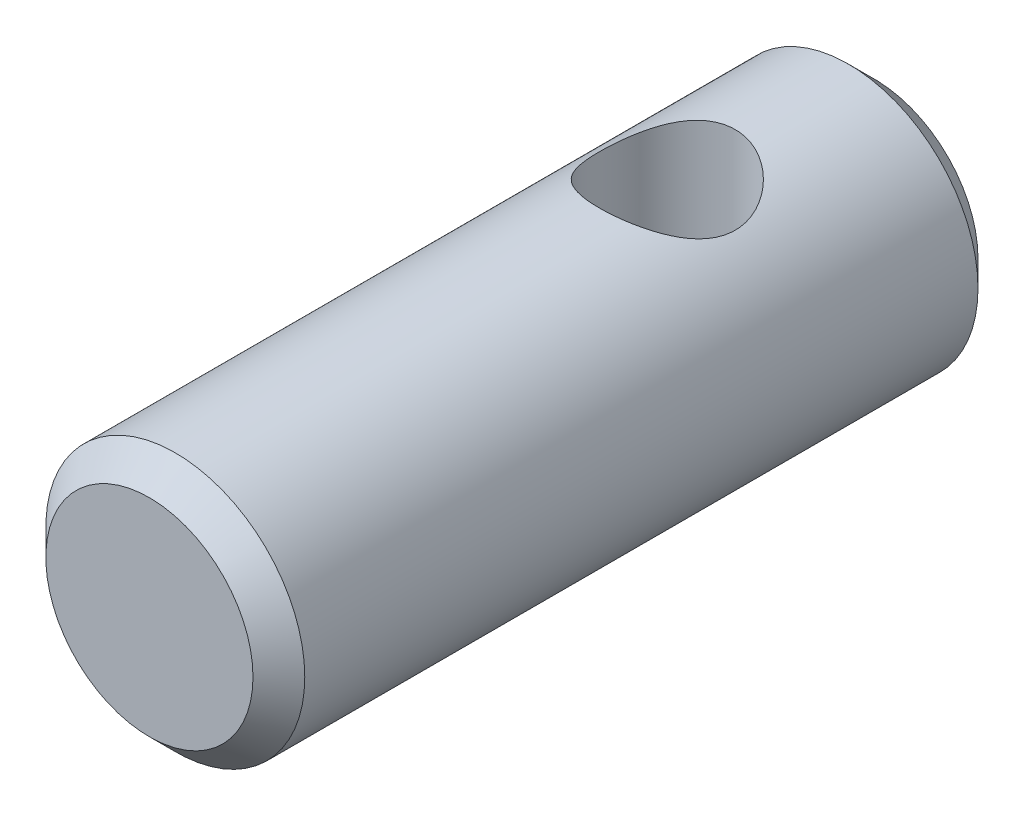
from build123d import *

# Parameters (mm, degrees)
PIN_PROFILE_20_R         = 10
PIN_BODY_20X56_DEPTH     = 56
CROSS_HOLE_SKETCH_10_5_R = 5.25
CROSS_HOLE_10_5_DEPTH    = 10
END_CHAMFER_2X45_SIZE    = 2


with BuildPart() as part:
    # Pin Profile Ø20 → Pin Body Ø20x56 (new body)
    with BuildSketch(Plane.XY):
        Circle(PIN_PROFILE_20_R)
    extrude(amount=PIN_BODY_20X56_DEPTH)

    # Cross Hole Sketch Ø10.5 → Cross Hole Ø10.5 (cut, symmetric)
    with BuildSketch(Plane(origin=(0, 0, 0), x_dir=(1, 0, 0), z_dir=(0, 1, 0))):
        with Locations(Location((0, -16, 0), (0, 0, 270))):
            Circle(CROSS_HOLE_SKETCH_10_5_R)
    extrude(amount=CROSS_HOLE_10_5_DEPTH, both=True, mode=Mode.SUBTRACT)

    # End Chamfer 2x45°
    end_chamfer_2x45_edges = [part.edges().sort_by_distance(p)[0] for p in [
        (-10, 0, 0),
        (-10, 0, 56),
    ]]
    chamfer(end_chamfer_2x45_edges, length=END_CHAMFER_2X45_SIZE)


solid = part.part
